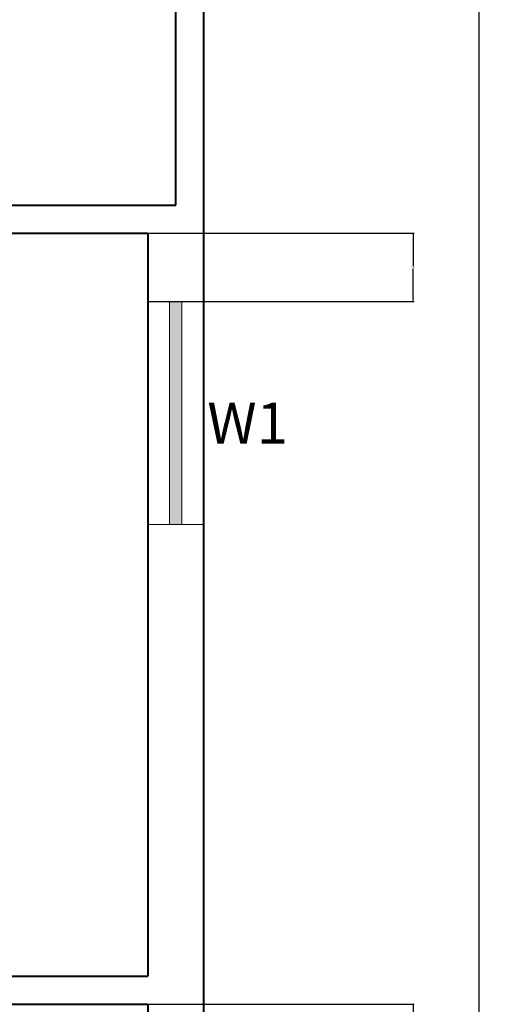
# Model space of a CAD drawing. Units: inches. Extents: x 182 to 1022, y -617 to 111.
# Tile 32 of 33: x 943 to 1022, y -246 to -87. Entities that reach past the tile are written whole.
import ezdxf

# ---------------------------------------------------------------- set-up
doc = ezdxf.new("R2010")
doc.units = ezdxf.units.IN
doc.header["$MEASUREMENT"] = 0
for name, color, linetype, lineweight in [('A-ANNO-DIMS', 2, 'Continuous', 18), ('A-ANNO-IDEN', 1, 'Continuous', 18), ('A-GLAZ-PATT', 5, 'Continuous', 13), ('wall', 1, 'Continuous', 40), ('wind', 5, 'Continuous', 20)]:
    doc.layers.add(name, color=color, linetype=linetype, lineweight=lineweight)
doc.styles.get("Standard").update_dxf_attribs({"font": 'arial.ttf'})
doc.dimstyles.get("Standard").update_dxf_attribs({"dimtxt": 0.18, "dimasz": 0.18, "dimexe": 0.18, "dimexo": 0.0625, "dimgap": 0.09, "dimtad": 0, "dimtih": 1, "dimtoh": 1, "dimdec": 1, "dimzin": 0, "dimdsep": 46, "dimlunit": 4, "dimtxsty": 'Standard', "dimcen": 0.09, "dimadec": 0, "dimazin": 0, "dimtfac": 1, "dimtdec": 1, "dimtofl": 0, "dimtmove": 0, "dimatfit": 3, "dimfxl": 1, "dimtolj": 1, "dimtzin": 0, "dimarcsym": 0})

# ---------------------------------------------------------------- blocks, each defined once
blk = doc.blocks.new('_ArchTick')
at = {"color": 0, "linetype": 'ByBlock', "const_width": 0.15}
blk.add_lwpolyline([(-0.5, -0.5), (0.5, 0.5)], dxfattribs=at)
blk = doc.blocks.new('*D8')
at = {"layer": 'A-ANNO-DIMS', "color": 0, "lineweight": -2, "transparency": 16777216}
for p, q in [((1016.69, -0.37), (1016.69, -260.42)), ((1016.69, -540.37), (1016.69, -280.32))]:
    blk.add_line(p, q, dxfattribs=at)
at = {"layer": 'Defpoints', "color": 0, "transparency": 16777216}
for p in [(972.3, -0.37), (972.3, -540.37), (1016.69, -540.37)]:
    blk.add_point(p, dxfattribs=at)
at = {"layer": 'A-ANNO-DIMS', "color": 0, "lineweight": -2, "transparency": 16777216, "xscale": 8, "yscale": 8, "zscale": 8}
for p, rotation in [((1016.69, -0.37), 90), ((1016.69, -540.37), 270)]:
    blk.add_blockref('_ArchTick', p, dxfattribs=dict(at, rotation=rotation))
at = {"layer": 'A-ANNO-DIMS', "color": 0, "transparency": 16777216, "insert": (1016.69, -270.37), "char_height": 8, "attachment_point": 5, "rotation": 90}
blk.add_mtext("\\A1;45'", dxfattribs=at)
blk = doc.blocks.new('*D36')
at = {"layer": 'A-ANNO-DIMS', "color": 0, "lineweight": -2, "transparency": 16777216}
for p, q in [((963.37, -121.87), (1006.28, -121.87)), ((1006.1, -122.05), (1006.1, -127.21)), ((1006.1, -132.74), (1006.1, -127.58)), ((963.37, -132.92), (1006.28, -132.92))]:
    blk.add_line(p, q, dxfattribs=at)
at = {"layer": 'A-ANNO-DIMS', "color": 0, "transparency": 16777216}
for points in [[(1006.07, -122.05), (1006.13, -122.05), (1006.1, -121.87)], [(1006.07, -132.74), (1006.13, -132.74), (1006.1, -132.92)]]:
    blk.add_solid(points, dxfattribs=at)
at = {"layer": 'Defpoints', "color": 0, "transparency": 16777216}
for p in [(963.3, -121.87), (963.3, -132.92), (1006.1, -132.92)]:
    blk.add_point(p, dxfattribs=at)
at = {"layer": 'A-ANNO-DIMS', "color": 0, "transparency": 16777216, "insert": (1006.1, -127.4), "char_height": 0.18, "attachment_point": 5}
blk.add_mtext('\\A1;0\'-11"', dxfattribs=at)
blk = doc.blocks.new('*D37')
at = {"layer": 'A-ANNO-DIMS', "color": 0, "lineweight": -2, "transparency": 16777216}
for p, q in [((963.37, -246.37), (1006.28, -246.37)), ((1006.1, -246.55), (1006.1, -252.19)), ((1006.1, -258.19), (1006.1, -252.56)), ((963.37, -258.37), (1006.28, -258.37))]:
    blk.add_line(p, q, dxfattribs=at)
at = {"layer": 'A-ANNO-DIMS', "color": 0, "transparency": 16777216}
for points in [[(1006.07, -246.55), (1006.13, -246.55), (1006.1, -246.37)], [(1006.07, -258.19), (1006.13, -258.19), (1006.1, -258.37)]]:
    blk.add_solid(points, dxfattribs=at)
at = {"layer": 'Defpoints', "color": 0, "transparency": 16777216}
for p in [(963.3, -246.37), (963.3, -258.37), (1006.1, -258.37)]:
    blk.add_point(p, dxfattribs=at)
at = {"layer": 'A-ANNO-DIMS', "color": 0, "transparency": 16777216, "insert": (1006.1, -252.37), "char_height": 0.18, "attachment_point": 5}
blk.add_mtext('\\A1;1\'-0"', dxfattribs=at)

msp = doc.modelspace()

# ---------------------------------------------------------------- hatches: boundary and pattern name
at = {"layer": 'A-GLAZ-PATT'}
h = msp.add_hatch(color=256, dxfattribs=at)
h.dxf.hatch_style = 1
h.paths.add_polyline_path([(692.35, -3.87), (662.35, -3.87), (662.35, -5.87), (692.35, -5.87)])
h.paths.add_polyline_path([(783.03, -3.87), (747.03, -3.87), (747.03, -5.87), (783.03, -5.87)])
h.paths.add_polyline_path([(641.8, -252.37), (639.8, -252.37), (639.8, -288.37), (641.8, -288.37)])
h.paths.add_polyline_path([(968.8, -258.37), (966.8, -258.37), (966.8, -282.37), (968.8, -282.37)])
h.paths.add_polyline_path([(968.8, -132.92), (966.8, -132.92), (966.8, -168.92), (968.8, -168.92)])
h.paths.add_polyline_path([(940.3, -534.87), (904.3, -534.87), (904.3, -536.87), (940.3, -536.87)])

# ---------------------------------------------------------------- linework, layer by layer
at = {"layer": 'wall'}
for p, q in [((972.3, -540.37), (972.3, -0.37)), ((967.8, -117.37), (967.8, -4.87)), ((835.8, -117.37), (967.8, -117.37)), ((840.3, -121.87), (963.3, -121.87)), ((963.3, -121.87), (963.3, -241.87)), ((876.3, -241.87), (963.3, -241.87)), ((876.3, -246.37), (963.3, -246.37)), ((963.3, -246.37), (963.3, -318.37))]:
    msp.add_line(p, q, dxfattribs=at)
at = {"layer": 'wind'}
for p, q in [((963.3, -132.92), (972.3, -132.92)), ((966.8, -132.92), (966.8, -168.92)), ((968.8, -132.92), (968.8, -168.92)), ((963.3, -168.92), (972.3, -168.92))]:
    msp.add_line(p, q, dxfattribs=at)

# ---------------------------------------------------------------- texts
at = {"layer": 'A-ANNO-IDEN'}
msp.add_text('W1', height=6.652, dxfattribs=at).set_placement((972.88, -155.89))

# ---------------------------------------------------------------- dimensions: what is measured, and where the dimension line sits
at = {"layer": 'A-ANNO-DIMS'}
for base, p1, p2, angle, override, picture, middle in [((1016.69, -540.37), (972.3, -0.37), (972.3, -540.37), 90, {"dimtxt": 8, "dimasz": 8, "dimgap": 3, "dimtih": 0, "dimblk1": 'ArchTick', "dimblk2": 'ArchTick', "dimsah": 1, "dimse1": 1, "dimse2": 1, "dimclrd": 0, "dimclre": 0, "dimclrt": 0}, '*D8', (1016.69, -270.37)), ((1006.1048, -132.9203), (963.3048, -121.8732), (963.3048, -132.9203), 270, {"dimdec": 1, "dimlfac": 1, "dimrnd": 0, "dimzin": 1, "dimdsep": 46, "dimlunit": 4, "dimfrac": 2}, '*D36', (1006.1048, -127.3967)), ((1006.1, -258.37), (963.3, -246.37), (963.3, -258.37), 270, {"dimdec": 1, "dimlfac": 1, "dimrnd": 0, "dimzin": 1, "dimdsep": 46, "dimlunit": 4, "dimfrac": 2}, '*D37', (1006.1, -252.37))]:
    dim = msp.add_linear_dim(base=base, p1=p1, p2=p2, angle=angle, dimstyle='Standard', override=override, dxfattribs=at)
    dim.commit()
    dim.dimension.update_dxf_attribs({"geometry": picture, "text_midpoint": middle})

doc.saveas('drawing.dxf')
